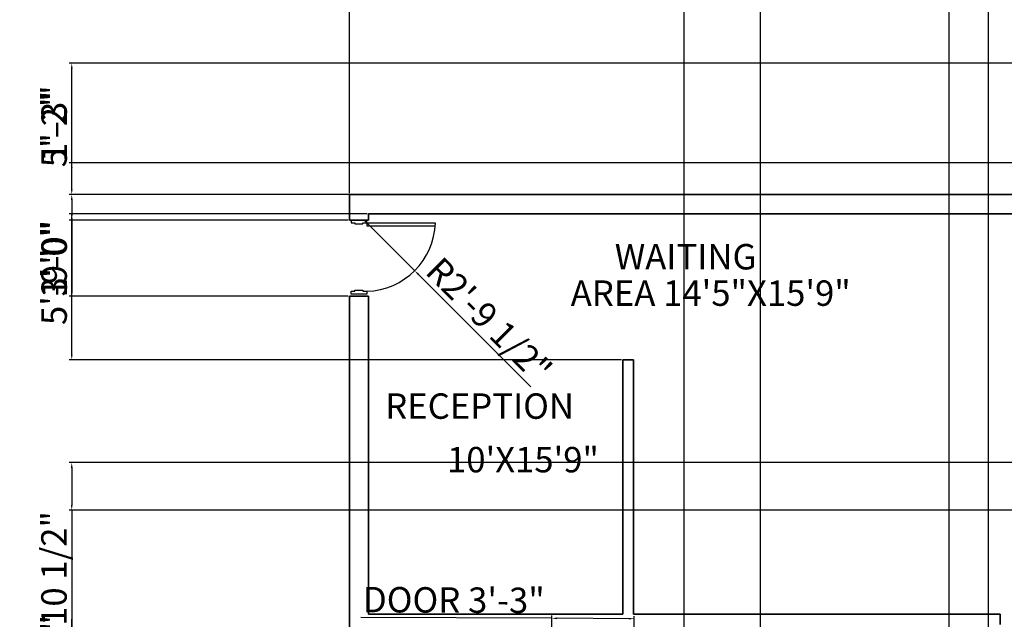
# Model space of a CAD drawing. Units: inches. Extents: x 2319 to 3765, y 2872 to 3950.
# Tile 4 of 9: x 2319 to 2783, y 3306 to 3589. Entities that reach past the tile are written whole.
import ezdxf

# ---------------------------------------------------------------- set-up
doc = ezdxf.new("R2010")
doc.units = ezdxf.units.IN
for name, color, linetype, lineweight in [('A-ANNO-DIMS', 2, 'Continuous', 18), ('A-AREA-IDEN', 7, 'Continuous', 18), ('A-DOOR', 3, 'Continuous', 25), ('A-WALL', 7, 'Continuous', 35)]:
    doc.layers.add(name, color=color, linetype=linetype, lineweight=lineweight)
doc.styles.get("Standard").update_dxf_attribs({"font": 'arial.ttf'})
doc.dimstyles.new('ISO-25', dxfattribs={"dimtxt": 12, "dimasz": 2.5, "dimexe": 1.25, "dimexo": 0.625, "dimtad": 1, "dimdec": 0, "dimlunit": 3, "dimtxsty": 'Standard', "dimcen": 2.5, "dimadec": 0, "dimazin": 0, "dimtfac": 1, "dimtdec": 0, "dimtmove": 0, "dimatfit": 3, "dimfxl": 1, "dimarcsym": 0})

# ---------------------------------------------------------------- blocks, each defined once
blk = doc.blocks.new('A$C769D55ED')
for p, q in [((34, 192), (34, 1025)), ((72, 192), (72, 1024)), ((0, 192), (0, 0)), ((34, 192), (0, 192)), ((34, 144), (34, 192)), ((48, 144), (34, 144)), ((48, 48), (48, 144)), ((34, 0), (34, 48)), ((34, 48), (48, 48)), ((0, 0), (34, 0))]:
    blk.add_line(p, q)
blk.add_lwpolyline([(34, 192), (72, 192)])
blk.add_lwpolyline([(900, 192), (900, 0), (866, 0), (866, 48), (852, 48), (852, 144), (866, 144), (866, 192)], close=True)
blk.add_arc((7, 166), 860, 1.7624, 88.2376)
blk = doc.blocks.new('*D55')
at = {"layer": 'A-ANNO-DIMS', "color": 0, "lineweight": -2, "transparency": 16777216}
for p, q in [((2569.58, 3301.38), (2569.62, 3307.84)), ((2608.46, 3301.19), (2608.49, 3307.65)), ((2569.61, 3306.59), (2479.61, 3307.04)), ((2605.99, 3306.41), (2572.11, 3306.58))]:
    blk.add_line(p, q, dxfattribs=at)
at = {"layer": 'A-ANNO-DIMS', "color": 0, "transparency": 16777216}
for points in [[(2572.11, 3307), (2572.11, 3306.16), (2569.61, 3306.59)], [(2605.99, 3306.83), (2605.98, 3305.99), (2608.49, 3306.4)]]:
    blk.add_solid(points, dxfattribs=at)
at = {"layer": 'Defpoints', "color": 0, "transparency": 16777216}
for p in [(2569.61, 3306.59), (2569.58, 3300.76), (2608.46, 3300.57)]:
    blk.add_point(p, dxfattribs=at)
at = {"layer": 'A-ANNO-DIMS', "color": 0, "transparency": 16777216, "insert": (2523.39, 3313.66), "char_height": 12, "attachment_point": 5, "rotation": 359.7171}
blk.add_mtext('DOOR 3\'-3"', dxfattribs=at)
blk = doc.blocks.new('*D71')
at = {"layer": 'A-ANNO-DIMS', "color": 0, "lineweight": -2, "transparency": 16777216}
for p, q in [((2474.13, 3507.24), (2474.13, 3605.01)), ((2955.13, 3569.24), (2955.13, 3605.01)), ((2476.63, 3603.76), (2952.63, 3603.76))]:
    blk.add_line(p, q, dxfattribs=at)
at = {"layer": 'A-ANNO-DIMS', "color": 0, "transparency": 16777216}
for points in [[(2476.63, 3604.18), (2476.63, 3603.34), (2474.13, 3603.76)], [(2952.63, 3604.18), (2952.63, 3603.34), (2955.13, 3603.76)]]:
    blk.add_solid(points, dxfattribs=at)
at = {"layer": 'Defpoints', "color": 0, "transparency": 16777216}
for p in [(2955.13, 3603.76), (2955.13, 3568.61), (2474.13, 3506.61)]:
    blk.add_point(p, dxfattribs=at)
at = {"layer": 'A-ANNO-DIMS', "color": 0, "transparency": 16777216, "insert": (2714.63, 3610.51), "char_height": 12, "attachment_point": 5}
blk.add_mtext('40\'-1"', dxfattribs=at)
blk = doc.blocks.new('*D73')
at = {"layer": 'A-ANNO-DIMS', "color": 0, "lineweight": -2, "transparency": 16777216}
for p, q in [((2474.13, 3507.24), (2474.13, 3605.01)), ((2825.13, 3507.24), (2825.13, 3605.01)), ((2476.63, 3603.76), (2822.63, 3603.76))]:
    blk.add_line(p, q, dxfattribs=at)
at = {"layer": 'A-ANNO-DIMS', "color": 0, "transparency": 16777216}
for points in [[(2476.63, 3604.18), (2476.63, 3603.34), (2474.13, 3603.76)], [(2822.63, 3604.18), (2822.63, 3603.34), (2825.13, 3603.76)]]:
    blk.add_solid(points, dxfattribs=at)
at = {"layer": 'Defpoints', "color": 0, "transparency": 16777216}
for p in [(2825.13, 3603.76), (2474.13, 3506.61), (2825.13, 3506.61)]:
    blk.add_point(p, dxfattribs=at)
at = {"layer": 'A-ANNO-DIMS', "color": 0, "transparency": 16777216, "insert": (2649.63, 3610.52), "char_height": 12, "attachment_point": 5}
blk.add_mtext('29\'-3"', dxfattribs=at)
blk = doc.blocks.new('*D74')
at = {"layer": 'A-ANNO-DIMS', "color": 0, "lineweight": -2, "transparency": 16777216}
for p, q in [((2824.5, 3568.61), (2341.89, 3568.61)), ((2343.14, 3509.11), (2343.14, 3566.11)), ((2824.5, 3506.61), (2341.89, 3506.61))]:
    blk.add_line(p, q, dxfattribs=at)
at = {"layer": 'A-ANNO-DIMS', "color": 0, "transparency": 16777216}
for points in [[(2342.72, 3566.11), (2343.56, 3566.11), (2343.14, 3568.61)], [(2342.72, 3509.11), (2343.56, 3509.11), (2343.14, 3506.61)]]:
    blk.add_solid(points, dxfattribs=at)
at = {"layer": 'Defpoints', "color": 0, "transparency": 16777216}
for p in [(2343.14, 3568.61), (2825.13, 3568.61), (2825.13, 3506.61)]:
    blk.add_point(p, dxfattribs=at)
at = {"layer": 'A-ANNO-DIMS', "color": 0, "transparency": 16777216, "insert": (2336.39, 3537.61), "char_height": 12, "attachment_point": 5, "rotation": 90}
blk.add_mtext('5\'-2"', dxfattribs=at)
blk = doc.blocks.new('*D75')
at = {"layer": 'A-ANNO-DIMS', "color": 0, "lineweight": -2, "transparency": 16777216}
for p, q in [((2632.13, 2970.24), (2632.13, 3605.01)), ((2668.13, 2970.24), (2668.13, 3605.01)), ((2634.63, 3603.76), (2665.63, 3603.76))]:
    blk.add_line(p, q, dxfattribs=at)
at = {"layer": 'A-ANNO-DIMS', "color": 0, "transparency": 16777216}
for points in [[(2634.63, 3604.18), (2634.63, 3603.34), (2632.13, 3603.76)], [(2665.63, 3604.18), (2665.63, 3603.34), (2668.13, 3603.76)]]:
    blk.add_solid(points, dxfattribs=at)
at = {"layer": 'Defpoints', "color": 0, "transparency": 16777216}
for p in [(2668.13, 3603.76), (2632.13, 2969.61), (2668.13, 2969.61)]:
    blk.add_point(p, dxfattribs=at)
at = {"layer": 'A-ANNO-DIMS', "color": 0, "transparency": 16777216, "insert": (2650.13, 3610.52), "char_height": 12, "attachment_point": 5}
blk.add_mtext('3\'-0"', dxfattribs=at)
blk = doc.blocks.new('*D76')
at = {"layer": 'A-ANNO-DIMS', "color": 0, "lineweight": -2, "transparency": 16777216}
for p, q in [((2757.13, 2970.24), (2757.13, 3605.01)), ((2775.67, 2970.24), (2775.67, 3605.01)), ((2759.63, 3603.76), (2773.17, 3603.76)), ((2775.67, 3603.76), (2838.15, 3603.76))]:
    blk.add_line(p, q, dxfattribs=at)
at = {"layer": 'A-ANNO-DIMS', "color": 0, "transparency": 16777216}
for points in [[(2759.63, 3604.18), (2759.63, 3603.34), (2757.13, 3603.76)], [(2773.17, 3604.18), (2773.17, 3603.34), (2775.67, 3603.76)]]:
    blk.add_solid(points, dxfattribs=at)
at = {"layer": 'Defpoints', "color": 0, "transparency": 16777216}
for p in [(2775.67, 3603.76), (2757.13, 2969.61), (2775.67, 2969.61)]:
    blk.add_point(p, dxfattribs=at)
at = {"layer": 'A-ANNO-DIMS', "color": 0, "transparency": 16777216, "insert": (2808.16, 3610.59), "char_height": 12, "attachment_point": 5}
blk.add_mtext('1\'-6 1/2"', dxfattribs=at)
blk = doc.blocks.new('*D83')
at = {"layer": 'A-ANNO-DIMS', "color": 0, "lineweight": -2, "transparency": 16777216}
for p, q in [((2473.5, 3506.61), (2341.89, 3506.61)), ((2343.14, 3504.11), (2343.14, 3497.11)), ((2473.5, 3494.61), (2341.89, 3494.61)), ((2343.14, 3494.61), (2343.14, 3460.09))]:
    blk.add_line(p, q, dxfattribs=at)
at = {"layer": 'A-ANNO-DIMS', "color": 0, "transparency": 16777216}
for points in [[(2342.72, 3504.11), (2343.56, 3504.11), (2343.14, 3506.61)], [(2342.72, 3497.11), (2343.56, 3497.11), (2343.14, 3494.61)]]:
    blk.add_solid(points, dxfattribs=at)
at = {"layer": 'Defpoints', "color": 0, "transparency": 16777216}
for p in [(2474.13, 3506.61), (2343.14, 3494.61), (2474.13, 3494.61)]:
    blk.add_point(p, dxfattribs=at)
at = {"layer": 'A-ANNO-DIMS', "color": 0, "transparency": 16777216, "insert": (2336.39, 3476.1), "char_height": 12, "attachment_point": 5, "rotation": 90}
blk.add_mtext('1\'-0"', dxfattribs=at)
blk = doc.blocks.new('*D84')
at = {"layer": 'A-ANNO-DIMS', "color": 0, "lineweight": -2, "transparency": 16777216}
for p, q in [((2473.5, 3494.61), (2341.89, 3494.61)), ((2343.14, 3492.11), (2343.14, 3461.11)), ((2473.5, 3458.61), (2341.89, 3458.61))]:
    blk.add_line(p, q, dxfattribs=at)
at = {"layer": 'A-ANNO-DIMS', "color": 0, "transparency": 16777216}
for points in [[(2342.72, 3492.11), (2343.56, 3492.11), (2343.14, 3494.61)], [(2342.72, 3461.11), (2343.56, 3461.11), (2343.14, 3458.61)]]:
    blk.add_solid(points, dxfattribs=at)
at = {"layer": 'Defpoints', "color": 0, "transparency": 16777216}
for p in [(2474.13, 3494.61), (2343.14, 3458.61), (2474.13, 3458.61)]:
    blk.add_point(p, dxfattribs=at)
at = {"layer": 'A-ANNO-DIMS', "color": 0, "transparency": 16777216, "insert": (2336.38, 3476.61), "char_height": 12, "attachment_point": 5, "rotation": 90}
blk.add_mtext('3\'-0"', dxfattribs=at)
blk = doc.blocks.new('*D85')
at = {"layer": 'A-ANNO-DIMS', "color": 0, "lineweight": -2, "transparency": 16777216}
for p, q in [((2482.5, 3497.61), (2341.89, 3497.61)), ((2343.14, 3431.11), (2343.14, 3495.11)), ((2602.5, 3428.61), (2341.89, 3428.61))]:
    blk.add_line(p, q, dxfattribs=at)
at = {"layer": 'A-ANNO-DIMS', "color": 0, "transparency": 16777216}
for points in [[(2342.72, 3495.11), (2343.56, 3495.11), (2343.14, 3497.61)], [(2342.72, 3431.11), (2343.56, 3431.11), (2343.14, 3428.61)]]:
    blk.add_solid(points, dxfattribs=at)
at = {"layer": 'Defpoints', "color": 0, "transparency": 16777216}
for p in [(2343.14, 3497.61), (2483.13, 3497.61), (2603.13, 3428.61)]:
    blk.add_point(p, dxfattribs=at)
at = {"layer": 'A-ANNO-DIMS', "color": 0, "transparency": 16777216, "insert": (2336.39, 3463.11), "char_height": 12, "attachment_point": 5, "rotation": 90}
blk.add_mtext('5\'-9"', dxfattribs=at)
blk = doc.blocks.new('*D86')
at = {"layer": 'A-ANNO-DIMS', "color": 0, "lineweight": -2, "transparency": 16777216}
for p, q in [((2343.14, 3521.62), (2343.14, 3556.13)), ((2824.5, 3521.62), (2341.89, 3521.62)), ((2343.14, 3509.11), (2343.14, 3519.12)), ((2824.5, 3506.61), (2341.89, 3506.61))]:
    blk.add_line(p, q, dxfattribs=at)
at = {"layer": 'A-ANNO-DIMS', "color": 0, "transparency": 16777216}
for points in [[(2342.72, 3519.12), (2343.56, 3519.12), (2343.14, 3521.62)], [(2342.72, 3509.11), (2343.56, 3509.11), (2343.14, 3506.61)]]:
    blk.add_solid(points, dxfattribs=at)
at = {"layer": 'Defpoints', "color": 0, "transparency": 16777216}
for p in [(2343.14, 3521.62), (2825.13, 3521.62), (2825.13, 3506.61)]:
    blk.add_point(p, dxfattribs=at)
at = {"layer": 'A-ANNO-DIMS', "color": 0, "transparency": 16777216, "insert": (2336.38, 3540.13), "char_height": 12, "attachment_point": 5, "rotation": 90}
blk.add_mtext('1\'-3"', dxfattribs=at)
blk = doc.blocks.new('*D87')
at = {"layer": 'A-ANNO-DIMS', "color": 0, "lineweight": -2, "transparency": 16777216}
for p, q in [((2800.5, 3380.11), (2341.89, 3380.11)), ((2343.14, 3377.61), (2343.14, 3360.11)), ((2800.5, 3357.61), (2341.89, 3357.61)), ((2343.14, 3357.61), (2343.14, 3285.81))]:
    blk.add_line(p, q, dxfattribs=at)
at = {"layer": 'A-ANNO-DIMS', "color": 0, "transparency": 16777216}
for points in [[(2342.72, 3377.61), (2343.56, 3377.61), (2343.14, 3380.11)], [(2342.72, 3360.11), (2343.56, 3360.11), (2343.14, 3357.61)]]:
    blk.add_solid(points, dxfattribs=at)
at = {"layer": 'Defpoints', "color": 0, "transparency": 16777216}
for p in [(2801.13, 3380.11), (2343.14, 3357.61), (2801.13, 3357.61)]:
    blk.add_point(p, dxfattribs=at)
at = {"layer": 'A-ANNO-DIMS', "color": 0, "transparency": 16777216, "insert": (2336.31, 3320.46), "char_height": 12, "attachment_point": 5, "rotation": 90}
blk.add_mtext('1\'-10 1/2"', dxfattribs=at)
blk = doc.blocks.new('*D88')
at = {"layer": 'A-ANNO-DIMS', "color": 0, "lineweight": -2, "transparency": 16777216}
for p, q in [((2343.14, 3271.61), (2343.14, 3306.13)), ((2949.5, 3271.61), (2341.89, 3271.61)), ((2343.14, 3256.11), (2343.14, 3269.11)), ((2949.5, 3253.61), (2341.89, 3253.61))]:
    blk.add_line(p, q, dxfattribs=at)
at = {"layer": 'A-ANNO-DIMS', "color": 0, "transparency": 16777216}
for points in [[(2342.72, 3269.11), (2343.56, 3269.11), (2343.14, 3271.61)], [(2342.72, 3256.11), (2343.56, 3256.11), (2343.14, 3253.61)]]:
    blk.add_solid(points, dxfattribs=at)
at = {"layer": 'Defpoints', "color": 0, "transparency": 16777216}
for p in [(2343.14, 3271.61), (2950.13, 3271.61), (2950.13, 3253.61)]:
    blk.add_point(p, dxfattribs=at)
at = {"layer": 'A-ANNO-DIMS', "color": 0, "transparency": 16777216, "insert": (2336.39, 3290.12), "char_height": 12, "attachment_point": 5, "rotation": 90}
blk.add_mtext('1\'-6"', dxfattribs=at)
blk = doc.blocks.new('*D103')
at = {"layer": 'A-ANNO-DIMS', "color": 0, "lineweight": -2, "transparency": 16777216}
for p, q in [((2481.33, 3494.33), (2504.92, 3470.74)), ((2559.78, 3415.87), (2506.68, 3468.97))]:
    blk.add_line(p, q, dxfattribs=at)
at = {"layer": 'A-ANNO-DIMS', "color": 0, "transparency": 16777216}
blk.add_solid([(2506.98, 3469.27), (2506.39, 3468.68), (2504.92, 3470.74)], dxfattribs=at)
at = {"layer": 'Defpoints', "color": 0, "transparency": 16777216}
for p in [(2481.33, 3494.33), (2504.92, 3470.74)]:
    blk.add_point(p, dxfattribs=at)
at = {"layer": 'A-ANNO-DIMS', "color": 0, "transparency": 16777216, "insert": (2538.95, 3446.37), "char_height": 12, "attachment_point": 5, "rotation": 314.9996}
blk.add_mtext('R2\'-9 1/2"', dxfattribs=at)

msp = doc.modelspace()

# ---------------------------------------------------------------- linework, layer by layer
at = {"layer": 'A-WALL'}
for p, q in [((2474.13, 3506.61), (2825.13, 3506.61)), ((2474.13, 3494.61), (2474.13, 3506.61)), ((2483.13, 3494.61), (2474.13, 3494.61)), ((2483.13, 3497.61), (2608.13, 3497.61)), ((2483.13, 3494.61), (2483.13, 3497.61)), ((2608.13, 3497.61), (2825.13, 3497.61)), ((2474.13, 2960.61), (2474.13, 3458.61)), ((2483.13, 3458.61), (2474.13, 3458.61)), ((2483.13, 3308.61), (2483.13, 3458.61)), ((2603.13, 3308.61), (2603.13, 3428.61)), ((2603.13, 3428.61), (2608.13, 3428.61)), ((2608.13, 3428.61), (2608.13, 3308.61)), ((2483.13, 3308.61), (2603.13, 3308.61)), ((2608.13, 3308.61), (2781.13, 3308.61)), ((2781.13, 3308.61), (2781.13, 3303.61))]:
    msp.add_line(p, q, dxfattribs=at)

# ---------------------------------------------------------------- block references
at = {"layer": 'A-DOOR', "xscale": 0.0388089662083284, "yscale": 0.0388089662083284, "zscale": 0.0388089662083284, "rotation": 270}
msp.add_blockref('A$C769D55ED', (2474.9, 3494.61), dxfattribs=at)

# ---------------------------------------------------------------- texts
at = {"layer": 'A-AREA-IDEN'}
for s, p in [('WAITING', (2599.34, 3471.29)), ('AREA 14\'5"X15\'9"', (2578.55, 3454.1)), ('RECEPTION ', (2491.04, 3400.77)), ('10\'X15\'9"', (2520.21, 3375.49))]:
    msp.add_text(s, height=12, dxfattribs=at).set_placement(p)

# ---------------------------------------------------------------- dimensions: what is measured, and where the dimension line sits
at = {"layer": 'A-ANNO-DIMS'}
for base, p1, p2, picture, middle in [((2775.67, 3603.76), (2757.13, 2969.61), (2775.67, 2969.61), '*D76', (2808.16, 3610.59)), ((2955.13, 3603.76), (2474.13, 3506.61), (2955.13, 3568.61), '*D71', (2714.63, 3610.51)), ((2825.13, 3603.76), (2474.13, 3506.61), (2825.13, 3506.61), '*D73', (2649.63, 3610.52)), ((2668.13, 3603.76), (2632.13, 2969.61), (2668.13, 2969.61), '*D75', (2650.13, 3610.52))]:
    dim = msp.add_linear_dim(base=base, p1=p1, p2=p2, dimstyle='ISO-25', override={"dimdec": 1, "dimlfac": 1, "dimrnd": 0, "dimzin": 1, "dimdsep": 46, "dimlunit": 4, "dimfrac": 2}, dxfattribs=at)
    dim.commit()
    dim.dimension.update_dxf_attribs({"geometry": picture, "text_midpoint": middle})
for base, p1, p2, picture, middle in [((2343.14, 3568.61), (2825.13, 3506.61), (2825.13, 3568.61), '*D74', (2336.39, 3537.61)), ((2343.14, 3521.62), (2825.13, 3506.61), (2825.13, 3521.62), '*D86', (2336.38, 3540.13)), ((2343.14, 3494.61), (2474.13, 3506.61), (2474.13, 3494.61), '*D83', (2336.39, 3476.1)), ((2343.14, 3497.61), (2603.13, 3428.61), (2483.13, 3497.61), '*D85', (2336.39, 3463.11)), ((2343.14, 3458.61), (2474.13, 3494.61), (2474.13, 3458.61), '*D84', (2336.38, 3476.61)), ((2343.14, 3357.61), (2801.13, 3380.11), (2801.13, 3357.61), '*D87', (2336.31, 3320.46)), ((2343.14, 3271.61), (2950.13, 3253.61), (2950.13, 3271.61), '*D88', (2336.39, 3290.12))]:
    dim = msp.add_linear_dim(base=base, p1=p1, p2=p2, angle=90, dimstyle='ISO-25', override={"dimdec": 1, "dimlfac": 1, "dimrnd": 0, "dimzin": 1, "dimdsep": 46, "dimlunit": 4, "dimfrac": 2}, dxfattribs=at)
    dim.commit()
    dim.dimension.update_dxf_attribs({"geometry": picture, "text_midpoint": middle})
dim = msp.add_radius_dim(center=(2481.33, 3494.33), mpoint=(2504.92, 3470.74), dimstyle='ISO-25', override={"dimdec": 1, "dimlfac": 1, "dimrnd": 0, "dimzin": 1, "dimdsep": 46, "dimlunit": 4, "dimfrac": 2}, dxfattribs=at)
dim.commit()
dim.dimension.update_dxf_attribs({"geometry": '*D103', "text_midpoint": (2538.95, 3446.37)})
dim = msp.add_linear_dim(base=(2569.61, 3306.59), p1=(2608.46, 3300.57), p2=(2569.58, 3300.76), angle=179.7171, text='DOOR <>', dimstyle='ISO-25', override={"dimdec": 1, "dimlfac": 1, "dimrnd": 0, "dimzin": 1, "dimdsep": 46, "dimlunit": 4, "dimfrac": 2}, dxfattribs=at)
dim.commit()
dim.dimension.update_dxf_attribs({"geometry": '*D55', "text_midpoint": (2523.39, 3313.66)})

doc.saveas('drawing.dxf')
